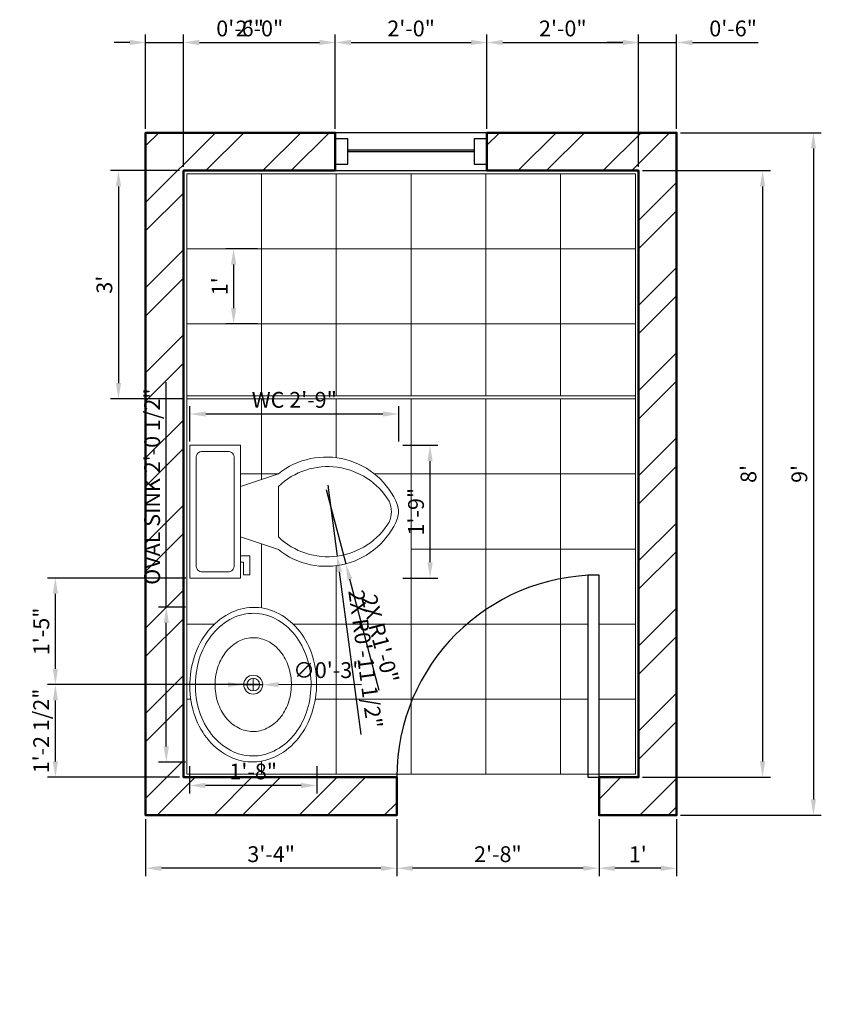
# Model space of a CAD drawing. Units: inches. Extents: x 3082 to 3209, y 1055 to 1366.
# Tile 2 of 2: x 3082 to 3209, y 1210 to 1366. Entities that reach past the tile are written whole.
import ezdxf

# ---------------------------------------------------------------- set-up
doc = ezdxf.new("R2010")
doc.units = ezdxf.units.IN
for name, color, linetype, lineweight in [('A-ANNO-DIMS', 2, 'Continuous', 18), ('A-DOOR', 3, 'Continuous', 25), ('A-FLOR-FIXT', 9, 'Continuous', 18), ('A-FLOR-PATT', 252, 'Continuous', 13), ('A-GLAZ', 4, 'Continuous', 25), ('A-WALL', 7, 'Continuous', 50), ('A-WALL-PATT', 8, 'Continuous', 13)]:
    doc.layers.add(name, color=color, linetype=linetype, lineweight=lineweight)
doc.styles.get("Standard").update_dxf_attribs({"font": 'arial.ttf'})
doc.dimstyles.new('ISO-25', dxfattribs={"dimtxt": 2.5, "dimasz": 2.5, "dimexe": 1.25, "dimexo": 0.625, "dimtad": 1, "dimdec": 0, "dimlunit": 3, "dimtxsty": 'Standard', "dimcen": 2.5, "dimadec": 0, "dimazin": 0, "dimtfac": 1, "dimtdec": 0, "dimtmove": 0, "dimatfit": 3, "dimfxl": 1, "dimarcsym": 0})

# ---------------------------------------------------------------- blocks, each defined once
blk = doc.blocks.new('*U2')
for p, q in [((0, 0), (0, -6)), ((-32, 0), (-32, -6))]:
    blk.add_line(p, q)
blk.add_lwpolyline([(0, 0), (0, 32), (-1.75, 32), (-1.75, 0)], close=True)
blk.add_arc((0, 0), 32, 90, 180)
blk = doc.blocks.new('Toilet - top')
for p, q in [((9.5, -6), (9.5, -2)), ((-10, -8.5), (-8, -8.5)), ((-10, -9.5), (-10, -8.5)), ((-8, -8.5), (-8, -8)), ((-7, -8), (-7, -9.5)), ((-4, -8), (-6, -14)), ((4, -8), (6, -14)), ((-7, -9.5), (-10, -9.5)), ((4, -14), (-4, -14))]:
    blk.add_line(p, q)
blk.add_lwpolyline([(10.5, -8), (10.5, 0), (-10.5, 0), (-10.5, -8)], close=True)
for points in [[(8.5, -1), (-8.5, -1)], [(-9.5, -2), (-9.5, -6)], [(-8.5, -7), (8.5, -7)]]:
    blk.add_lwpolyline(points)
for centre, radius, start, end in [((-8.62, -1.88), 0.884, 81.8699, 188.1301), ((8.62, -1.88), 0.884, 351.8699, 98.1301), ((-8.62, -6.12), 0.884, 171.8699, 278.1301), ((8.62, -6.12), 0.884, 261.8699, 8.1301), ((3.52, -21.58), 12.17, 141.4691, 247.9714), ((4.2, -21.82), 11.33, 136.3677, 238.9468), ((-3.52, -21.58), 12.17, 292.0284, 38.5307), ((-4.2, -21.82), 11.33, 301.053, 43.6321), ((0, -27.88), 4, 245.7318, 294.2682), ((0, -29), 4, 254.8605, 285.1395)]:
    blk.add_arc(centre, radius, start, end)
blk = doc.blocks.new('Sink - Oval top')
for p, q in [((-1, 0), (1, 0)), ((0, 1), (0, -1))]:
    blk.add_line(p, q)
for points in [[(-12.23, 0.39, 0.117634), (-11.46, -3.36, 0.104469), (-8.88, -6.8, 0.090016), (-5.08, -9.07, 0.08192), (-0.32, -10.02, 0.08192), (4.49, -9.38, 0.090016), (8.42, -7.36, 0.104469), (11.22, -4.09, 0.117634), (12.23, -0.39, 0.117634), (11.46, 3.36, 0.104469), (8.88, 6.8, 0.090016), (5.08, 9.07, 0.08192), (0.32, 10.02, 0.08192), (-4.49, 9.38, 0.090016), (-8.42, 7.36, 0.104469), (-11.22, 4.09, 0.117634)], [(-11.29, 0.16, 0.118622), (-10.52, -3.25, 0.104678), (-8.07, -6.36, 0.089562), (-4.54, -8.37, 0.081185), (-0.13, -9.15, 0.081185), (4.3, -8.49, 0.089562), (7.89, -6.58, 0.104678), (10.42, -3.55, 0.118622), (11.29, -0.16, 0.118622), (10.52, 3.25, 0.104678), (8.07, 6.36, 0.089562), (4.54, 8.37, 0.081185), (0.13, 9.15, 0.081185), (-4.3, 8.49, 0.089562), (-7.89, 6.58, 0.104678), (-10.42, 3.55, 0.118622)], [(-7.42, 0.08, 0.118283), (-6.91, -2.17, 0.104607), (-5.29, -4.21, 0.089718), (-2.97, -5.53, 0.081436), (-0.07, -6.04, 0.081436), (2.84, -5.59, 0.089718), (5.2, -4.33, 0.104607), (6.86, -2.32, 0.118283), (7.42, -0.08, 0.118283), (6.91, 2.17, 0.104607), (5.29, 4.21, 0.089718), (2.97, 5.53, 0.081436), (0.07, 6.04, 0.081436), (-2.84, 5.59, 0.089718), (-5.2, 4.33, 0.104607), (-6.86, 2.32, 0.118283)]]:
    blk.add_lwpolyline(points, format="xyb", close=True)
for radius in [1.5, 1]:
    blk.add_circle((0, 0), radius)
blk = doc.blocks.new('*D7')
at = {"layer": 'A-ANNO-DIMS', "color": 0, "lineweight": -2, "transparency": 16777216}
for p, q in [((3186.42, 1348.24), (3208.7, 1348.24)), ((3207.45, 1345.74), (3207.45, 1242.74)), ((3186.42, 1240.24), (3208.7, 1240.24))]:
    blk.add_line(p, q, dxfattribs=at)
at = {"layer": 'A-ANNO-DIMS', "color": 0, "transparency": 16777216}
for points in [[(3207.03, 1345.74), (3207.86, 1345.74), (3207.45, 1348.24)], [(3207.03, 1242.74), (3207.86, 1242.74), (3207.45, 1240.24)]]:
    blk.add_solid(points, dxfattribs=at)
at = {"layer": 'Defpoints', "color": 0, "transparency": 16777216}
for p in [(3185.8, 1348.24), (3185.8, 1240.24), (3207.45, 1240.24)]:
    blk.add_point(p, dxfattribs=at)
at = {"layer": 'A-ANNO-DIMS', "color": 0, "transparency": 16777216, "insert": (3205.55, 1294.24), "char_height": 2.5, "attachment_point": 5, "rotation": 90}
blk.add_mtext("9'", dxfattribs=at)
blk = doc.blocks.new('*D8')
at = {"layer": 'A-ANNO-DIMS', "color": 0, "lineweight": -2, "transparency": 16777216}
for p, q in [((3180.42, 1342.24), (3200.66, 1342.24)), ((3199.41, 1339.74), (3199.41, 1248.74)), ((3180.42, 1246.24), (3200.66, 1246.24))]:
    blk.add_line(p, q, dxfattribs=at)
at = {"layer": 'A-ANNO-DIMS', "color": 0, "transparency": 16777216}
for points in [[(3198.99, 1339.74), (3199.82, 1339.74), (3199.41, 1342.24)], [(3198.99, 1248.74), (3199.82, 1248.74), (3199.41, 1246.24)]]:
    blk.add_solid(points, dxfattribs=at)
at = {"layer": 'Defpoints', "color": 0, "transparency": 16777216}
for p in [(3179.8, 1342.24), (3179.8, 1246.24), (3199.41, 1246.24)]:
    blk.add_point(p, dxfattribs=at)
at = {"layer": 'A-ANNO-DIMS', "color": 0, "transparency": 16777216, "insert": (3197.5, 1294.24), "char_height": 2.5, "attachment_point": 5, "rotation": 90}
blk.add_mtext("8'", dxfattribs=at)
blk = doc.blocks.new('*D9')
at = {"layer": 'A-ANNO-DIMS', "color": 0, "lineweight": -2, "transparency": 16777216}
for p, q in [((3173.53, 1239.61), (3173.53, 1230.6)), ((3185.8, 1239.61), (3185.8, 1230.6)), ((3183.3, 1231.85), (3176.03, 1231.85))]:
    blk.add_line(p, q, dxfattribs=at)
at = {"layer": 'A-ANNO-DIMS', "color": 0, "transparency": 16777216}
for points in [[(3176.03, 1232.26), (3176.03, 1231.43), (3173.53, 1231.85)], [(3183.3, 1232.26), (3183.3, 1231.43), (3185.8, 1231.85)]]:
    blk.add_solid(points, dxfattribs=at)
at = {"layer": 'Defpoints', "color": 0, "transparency": 16777216}
for p in [(3173.53, 1240.24), (3185.8, 1240.24), (3173.53, 1231.85)]:
    blk.add_point(p, dxfattribs=at)
at = {"layer": 'A-ANNO-DIMS', "color": 0, "transparency": 16777216, "insert": (3179.66, 1233.73), "char_height": 2.5, "attachment_point": 5}
blk.add_mtext("1'", dxfattribs=at)
blk = doc.blocks.new('*D10')
at = {"layer": 'A-ANNO-DIMS', "color": 0, "lineweight": -2, "transparency": 16777216}
for p, q in [((3141.53, 1239.61), (3141.53, 1230.6)), ((3173.53, 1239.61), (3173.53, 1230.6)), ((3171.03, 1231.85), (3144.03, 1231.85))]:
    blk.add_line(p, q, dxfattribs=at)
at = {"layer": 'A-ANNO-DIMS', "color": 0, "transparency": 16777216}
for points in [[(3144.03, 1232.26), (3144.03, 1231.43), (3141.53, 1231.85)], [(3171.03, 1232.26), (3171.03, 1231.43), (3173.53, 1231.85)]]:
    blk.add_solid(points, dxfattribs=at)
at = {"layer": 'Defpoints', "color": 0, "transparency": 16777216}
for p in [(3141.53, 1240.24), (3173.53, 1240.24), (3141.53, 1231.85)]:
    blk.add_point(p, dxfattribs=at)
at = {"layer": 'A-ANNO-DIMS', "color": 0, "transparency": 16777216, "insert": (3157.53, 1233.75), "char_height": 2.5, "attachment_point": 5}
blk.add_mtext('2\'-8"', dxfattribs=at)
blk = doc.blocks.new('*D11')
at = {"layer": 'A-ANNO-DIMS', "color": 0, "lineweight": -2, "transparency": 16777216}
for p, q in [((3101.8, 1239.61), (3101.8, 1230.6)), ((3141.53, 1239.61), (3141.53, 1230.6)), ((3139.03, 1231.85), (3104.3, 1231.85))]:
    blk.add_line(p, q, dxfattribs=at)
at = {"layer": 'A-ANNO-DIMS', "color": 0, "transparency": 16777216}
for points in [[(3104.3, 1232.26), (3104.3, 1231.43), (3101.8, 1231.85)], [(3139.03, 1232.26), (3139.03, 1231.43), (3141.53, 1231.85)]]:
    blk.add_solid(points, dxfattribs=at)
at = {"layer": 'Defpoints', "color": 0, "transparency": 16777216}
for p in [(3101.8, 1240.24), (3141.53, 1240.24), (3101.8, 1231.85)]:
    blk.add_point(p, dxfattribs=at)
at = {"layer": 'A-ANNO-DIMS', "color": 0, "transparency": 16777216, "insert": (3121.66, 1233.75), "char_height": 2.5, "attachment_point": 5}
blk.add_mtext('3\'-4"', dxfattribs=at)
blk = doc.blocks.new('*D12')
at = {"layer": 'A-ANNO-DIMS', "color": 0, "lineweight": -2, "transparency": 16777216}
for p, q in [((3107.17, 1342.24), (3096.25, 1342.24)), ((3097.5, 1339.74), (3097.5, 1308.61)), ((3107.67, 1306.11), (3096.25, 1306.11))]:
    blk.add_line(p, q, dxfattribs=at)
at = {"layer": 'A-ANNO-DIMS', "color": 0, "transparency": 16777216}
for points in [[(3097.09, 1339.74), (3097.92, 1339.74), (3097.5, 1342.24)], [(3097.09, 1308.61), (3097.92, 1308.61), (3097.5, 1306.11)]]:
    blk.add_solid(points, dxfattribs=at)
at = {"layer": 'Defpoints', "color": 0, "transparency": 16777216}
for p in [(3107.8, 1342.24), (3097.5, 1306.11), (3108.3, 1306.11)]:
    blk.add_point(p, dxfattribs=at)
at = {"layer": 'A-ANNO-DIMS', "color": 0, "transparency": 16777216, "insert": (3095.6, 1324.18), "char_height": 2.5, "attachment_point": 5, "rotation": 90}
blk.add_mtext("3'", dxfattribs=at)
blk = doc.blocks.new('*D13')
at = {"layer": 'A-ANNO-DIMS', "color": 0, "lineweight": -2, "transparency": 16777216}
for p, q in [((3119.51, 1329.86), (3114.47, 1329.86)), ((3115.72, 1327.36), (3115.72, 1320.49)), ((3119.51, 1317.99), (3114.47, 1317.99))]:
    blk.add_line(p, q, dxfattribs=at)
at = {"layer": 'A-ANNO-DIMS', "color": 0, "transparency": 16777216}
for points in [[(3115.3, 1327.36), (3116.14, 1327.36), (3115.72, 1329.86)], [(3115.3, 1320.49), (3116.14, 1320.49), (3115.72, 1317.99)]]:
    blk.add_solid(points, dxfattribs=at)
at = {"layer": 'Defpoints', "color": 0, "transparency": 16777216}
for p in [(3120.13, 1329.86), (3115.72, 1317.99), (3120.13, 1317.99)]:
    blk.add_point(p, dxfattribs=at)
at = {"layer": 'A-ANNO-DIMS', "color": 0, "transparency": 16777216, "insert": (3113.84, 1323.93), "char_height": 2.5, "attachment_point": 5, "rotation": 90}
blk.add_mtext("1'", dxfattribs=at)
blk = doc.blocks.new('*D18')
at = {"layer": 'A-ANNO-DIMS', "color": 0, "lineweight": -2, "transparency": 16777216}
for p, q in [((3108.8, 1299.39), (3108.8, 1304.97)), ((3141.84, 1299.39), (3141.84, 1304.97)), ((3139.34, 1303.72), (3111.3, 1303.72))]:
    blk.add_line(p, q, dxfattribs=at)
at = {"layer": 'A-ANNO-DIMS', "color": 0, "transparency": 16777216}
for points in [[(3111.3, 1304.14), (3111.3, 1303.31), (3108.8, 1303.72)], [(3139.34, 1304.14), (3139.34, 1303.31), (3141.84, 1303.72)]]:
    blk.add_solid(points, dxfattribs=at)
at = {"layer": 'Defpoints', "color": 0, "transparency": 16777216}
for p in [(3108.8, 1303.72), (3108.8, 1298.77), (3141.84, 1298.77)]:
    blk.add_point(p, dxfattribs=at)
at = {"layer": 'A-ANNO-DIMS', "color": 0, "transparency": 16777216, "insert": (3125.32, 1305.64), "char_height": 2.5, "attachment_point": 5}
blk.add_mtext('WC 2\'-9"', dxfattribs=at)
blk = doc.blocks.new('*D19')
at = {"layer": 'A-ANNO-DIMS', "color": 0, "lineweight": -2, "transparency": 16777216}
for p, q in [((3142.47, 1298.77), (3148.05, 1298.77)), ((3146.8, 1280.27), (3146.8, 1296.27)), ((3142.47, 1277.77), (3148.05, 1277.77))]:
    blk.add_line(p, q, dxfattribs=at)
at = {"layer": 'A-ANNO-DIMS', "color": 0, "transparency": 16777216}
for points in [[(3146.38, 1296.27), (3147.22, 1296.27), (3146.8, 1298.77)], [(3146.38, 1280.27), (3147.22, 1280.27), (3146.8, 1277.77)]]:
    blk.add_solid(points, dxfattribs=at)
at = {"layer": 'Defpoints', "color": 0, "transparency": 16777216}
for p in [(3141.84, 1298.77), (3146.8, 1298.77), (3141.84, 1277.77)]:
    blk.add_point(p, dxfattribs=at)
at = {"layer": 'A-ANNO-DIMS', "color": 0, "transparency": 16777216, "insert": (3144.9, 1288.27), "char_height": 2.5, "attachment_point": 5, "rotation": 90}
blk.add_mtext('1\'-9"', dxfattribs=at)
blk = doc.blocks.new('*D20')
at = {"layer": 'A-ANNO-DIMS', "color": 0, "lineweight": -2, "transparency": 16777216}
for p, q in [((3105.07, 1273.17), (3105.07, 1308.78)), ((3108.13, 1273.17), (3103.82, 1273.17)), ((3105.07, 1251.12), (3105.07, 1270.67)), ((3108.13, 1248.62), (3103.82, 1248.62))]:
    blk.add_line(p, q, dxfattribs=at)
at = {"layer": 'A-ANNO-DIMS', "color": 0, "transparency": 16777216}
for points in [[(3104.65, 1270.67), (3105.49, 1270.67), (3105.07, 1273.17)], [(3104.65, 1251.12), (3105.49, 1251.12), (3105.07, 1248.62)]]:
    blk.add_solid(points, dxfattribs=at)
at = {"layer": 'Defpoints', "color": 0, "transparency": 16777216}
for p in [(3105.07, 1273.17), (3108.75, 1273.17), (3108.75, 1248.62)]:
    blk.add_point(p, dxfattribs=at)
at = {"layer": 'A-ANNO-DIMS', "color": 0, "transparency": 16777216, "insert": (3103.15, 1292.23), "char_height": 2.5, "attachment_point": 5, "rotation": 90}
blk.add_mtext('OVAL SINK 2\'-0 1/2"', dxfattribs=at)
blk = doc.blocks.new('*D21')
at = {"layer": 'A-ANNO-DIMS', "color": 0, "lineweight": -2, "transparency": 16777216}
for p, q in [((3108.75, 1248), (3108.75, 1243.69)), ((3128.89, 1248), (3128.89, 1243.69)), ((3126.39, 1244.94), (3111.25, 1244.94))]:
    blk.add_line(p, q, dxfattribs=at)
at = {"layer": 'A-ANNO-DIMS', "color": 0, "transparency": 16777216}
for points in [[(3111.25, 1245.36), (3111.25, 1244.52), (3108.75, 1244.94)], [(3126.39, 1245.36), (3126.39, 1244.52), (3128.89, 1244.94)]]:
    blk.add_solid(points, dxfattribs=at)
at = {"layer": 'Defpoints', "color": 0, "transparency": 16777216}
for p in [(3108.75, 1248.62), (3128.89, 1248.62), (3108.75, 1244.94)]:
    blk.add_point(p, dxfattribs=at)
at = {"layer": 'A-ANNO-DIMS', "color": 0, "transparency": 16777216, "insert": (3118.82, 1246.84), "char_height": 2.5, "attachment_point": 5}
blk.add_mtext('1\'-8"', dxfattribs=at)
blk = doc.blocks.new('*D24')
at = {"layer": 'A-ANNO-DIMS', "color": 0, "lineweight": -2, "transparency": 16777216}
for p, q in [((3101.8, 1348.86), (3101.8, 1363.76)), ((3107.8, 1342.86), (3107.8, 1363.76)), ((3099.3, 1362.51), (3096.8, 1362.51)), ((3101.8, 1362.51), (3107.8, 1362.51)), ((3110.3, 1362.51), (3120.69, 1362.51))]:
    blk.add_line(p, q, dxfattribs=at)
at = {"layer": 'A-ANNO-DIMS', "color": 0, "transparency": 16777216}
for points in [[(3099.3, 1362.93), (3099.3, 1362.1), (3101.8, 1362.51)], [(3110.3, 1362.93), (3110.3, 1362.1), (3107.8, 1362.51)]]:
    blk.add_solid(points, dxfattribs=at)
at = {"layer": 'Defpoints', "color": 0, "transparency": 16777216}
for p in [(3107.8, 1362.51), (3101.8, 1348.24), (3107.8, 1342.24)]:
    blk.add_point(p, dxfattribs=at)
at = {"layer": 'A-ANNO-DIMS', "color": 0, "transparency": 16777216, "insert": (3116.74, 1364.41), "char_height": 2.5, "attachment_point": 5}
blk.add_mtext('0\'-6"', dxfattribs=at)
blk = doc.blocks.new('*D25')
at = {"layer": 'A-ANNO-DIMS', "color": 0, "lineweight": -2, "transparency": 16777216}
for p, q in [((3107.8, 1342.86), (3107.8, 1363.76)), ((3131.8, 1348.86), (3131.8, 1363.76)), ((3110.3, 1362.51), (3129.3, 1362.51))]:
    blk.add_line(p, q, dxfattribs=at)
at = {"layer": 'A-ANNO-DIMS', "color": 0, "transparency": 16777216}
for points in [[(3110.3, 1362.93), (3110.3, 1362.1), (3107.8, 1362.51)], [(3129.3, 1362.93), (3129.3, 1362.1), (3131.8, 1362.51)]]:
    blk.add_solid(points, dxfattribs=at)
at = {"layer": 'Defpoints', "color": 0, "transparency": 16777216}
for p in [(3131.8, 1362.51), (3131.8, 1348.24), (3107.8, 1342.24)]:
    blk.add_point(p, dxfattribs=at)
at = {"layer": 'A-ANNO-DIMS', "color": 0, "transparency": 16777216, "insert": (3119.8, 1364.41), "char_height": 2.5, "attachment_point": 5}
blk.add_mtext('2\'-0"', dxfattribs=at)
blk = doc.blocks.new('*D26')
at = {"layer": 'A-ANNO-DIMS', "color": 0, "lineweight": -2, "transparency": 16777216}
for p, q in [((3131.8, 1348.86), (3131.8, 1363.76)), ((3155.8, 1348.86), (3155.8, 1363.76)), ((3134.3, 1362.51), (3153.3, 1362.51))]:
    blk.add_line(p, q, dxfattribs=at)
at = {"layer": 'A-ANNO-DIMS', "color": 0, "transparency": 16777216}
for points in [[(3134.3, 1362.93), (3134.3, 1362.1), (3131.8, 1362.51)], [(3153.3, 1362.93), (3153.3, 1362.1), (3155.8, 1362.51)]]:
    blk.add_solid(points, dxfattribs=at)
at = {"layer": 'Defpoints', "color": 0, "transparency": 16777216}
for p in [(3155.8, 1362.51), (3131.8, 1348.24), (3155.8, 1348.24)]:
    blk.add_point(p, dxfattribs=at)
at = {"layer": 'A-ANNO-DIMS', "color": 0, "transparency": 16777216, "insert": (3143.8, 1364.41), "char_height": 2.5, "attachment_point": 5}
blk.add_mtext('2\'-0"', dxfattribs=at)
blk = doc.blocks.new('*D27')
at = {"layer": 'A-ANNO-DIMS', "color": 0, "lineweight": -2, "transparency": 16777216}
for p, q in [((3155.8, 1348.86), (3155.8, 1363.76)), ((3179.8, 1342.86), (3179.8, 1363.76)), ((3158.3, 1362.51), (3177.3, 1362.51))]:
    blk.add_line(p, q, dxfattribs=at)
at = {"layer": 'A-ANNO-DIMS', "color": 0, "transparency": 16777216}
for points in [[(3158.3, 1362.93), (3158.3, 1362.1), (3155.8, 1362.51)], [(3177.3, 1362.93), (3177.3, 1362.1), (3179.8, 1362.51)]]:
    blk.add_solid(points, dxfattribs=at)
at = {"layer": 'Defpoints', "color": 0, "transparency": 16777216}
for p in [(3179.8, 1362.51), (3155.8, 1348.24), (3179.8, 1342.24)]:
    blk.add_point(p, dxfattribs=at)
at = {"layer": 'A-ANNO-DIMS', "color": 0, "transparency": 16777216, "insert": (3167.8, 1364.41), "char_height": 2.5, "attachment_point": 5}
blk.add_mtext('2\'-0"', dxfattribs=at)
blk = doc.blocks.new('*D28')
at = {"layer": 'A-ANNO-DIMS', "color": 0, "lineweight": -2, "transparency": 16777216}
for p, q in [((3179.8, 1342.86), (3179.8, 1363.76)), ((3185.8, 1348.86), (3185.8, 1363.76)), ((3177.3, 1362.51), (3174.8, 1362.51)), ((3179.8, 1362.51), (3185.8, 1362.51)), ((3188.3, 1362.51), (3198.69, 1362.51))]:
    blk.add_line(p, q, dxfattribs=at)
at = {"layer": 'A-ANNO-DIMS', "color": 0, "transparency": 16777216}
for points in [[(3177.3, 1362.93), (3177.3, 1362.1), (3179.8, 1362.51)], [(3188.3, 1362.93), (3188.3, 1362.1), (3185.8, 1362.51)]]:
    blk.add_solid(points, dxfattribs=at)
at = {"layer": 'Defpoints', "color": 0, "transparency": 16777216}
for p in [(3185.8, 1362.51), (3185.8, 1348.24), (3179.8, 1342.24)]:
    blk.add_point(p, dxfattribs=at)
at = {"layer": 'A-ANNO-DIMS', "color": 0, "transparency": 16777216, "insert": (3194.74, 1364.41), "char_height": 2.5, "attachment_point": 5}
blk.add_mtext('0\'-6"', dxfattribs=at)
blk = doc.blocks.new('*D29')
at = {"layer": 'A-ANNO-DIMS', "color": 0, "lineweight": -2, "transparency": 16777216}
for p, q in [((3119.7, 1260.9), (3086.27, 1260.9)), ((3087.52, 1248.74), (3087.52, 1258.4)), ((3107.17, 1246.24), (3086.27, 1246.24))]:
    blk.add_line(p, q, dxfattribs=at)
at = {"layer": 'A-ANNO-DIMS', "color": 0, "transparency": 16777216}
for points in [[(3087.11, 1258.4), (3087.94, 1258.4), (3087.52, 1260.9)], [(3087.11, 1248.74), (3087.94, 1248.74), (3087.52, 1246.24)]]:
    blk.add_solid(points, dxfattribs=at)
at = {"layer": 'Defpoints', "color": 0, "transparency": 16777216}
for p in [(3087.52, 1260.9), (3120.32, 1260.9), (3107.8, 1246.24)]:
    blk.add_point(p, dxfattribs=at)
at = {"layer": 'A-ANNO-DIMS', "color": 0, "transparency": 16777216, "insert": (3085.6, 1253.57), "char_height": 2.5, "attachment_point": 5, "rotation": 90}
blk.add_mtext('1\'-2 1/2"', dxfattribs=at)
blk = doc.blocks.new('*D30')
at = {"layer": 'A-ANNO-DIMS', "color": 0, "lineweight": -2, "transparency": 16777216}
for p, q in [((3108.17, 1277.77), (3086.27, 1277.77)), ((3087.52, 1263.4), (3087.52, 1275.27)), ((3119.7, 1260.9), (3086.27, 1260.9))]:
    blk.add_line(p, q, dxfattribs=at)
at = {"layer": 'A-ANNO-DIMS', "color": 0, "transparency": 16777216}
for points in [[(3087.11, 1275.27), (3087.94, 1275.27), (3087.52, 1277.77)], [(3087.11, 1263.4), (3087.94, 1263.4), (3087.52, 1260.9)]]:
    blk.add_solid(points, dxfattribs=at)
at = {"layer": 'Defpoints', "color": 0, "transparency": 16777216}
for p in [(3087.52, 1277.77), (3108.8, 1277.77), (3120.32, 1260.9)]:
    blk.add_point(p, dxfattribs=at)
at = {"layer": 'A-ANNO-DIMS', "color": 0, "transparency": 16777216, "insert": (3085.62, 1269.33), "char_height": 2.5, "attachment_point": 5, "rotation": 90}
blk.add_mtext('1\'-5"', dxfattribs=at)
blk = doc.blocks.new('*D41')
at = {"layer": 'A-ANNO-DIMS', "color": 0, "lineweight": -2, "transparency": 16777216}
for p, q in [((3130.38, 1291.79), (3133.47, 1280.02)), ((3138.73, 1259.99), (3134.11, 1277.6))]:
    blk.add_line(p, q, dxfattribs=at)
at = {"layer": 'A-ANNO-DIMS', "color": 0, "transparency": 16777216}
blk.add_solid([(3134.51, 1277.7), (3133.7, 1277.49), (3133.47, 1280.02)], dxfattribs=at)
at = {"layer": 'Defpoints', "color": 0, "transparency": 16777216}
for p in [(3130.38, 1291.79), (3133.47, 1280.02)]:
    blk.add_point(p, dxfattribs=at)
at = {"layer": 'A-ANNO-DIMS', "color": 0, "transparency": 16777216, "insert": (3138.57, 1268.07), "char_height": 2.5, "attachment_point": 5, "rotation": 284.7218}
blk.add_mtext('2X R1\'-0"', dxfattribs=at)
blk = doc.blocks.new('*D42')
at = {"layer": 'A-ANNO-DIMS', "color": 0, "lineweight": -2, "transparency": 16777216}
for p, q in [((3130.61, 1292.47), (3132.12, 1281.24)), ((3135.92, 1253.02), (3132.46, 1278.76))]:
    blk.add_line(p, q, dxfattribs=at)
at = {"layer": 'A-ANNO-DIMS', "color": 0, "transparency": 16777216}
blk.add_solid([(3132.87, 1278.82), (3132.04, 1278.71), (3132.12, 1281.24)], dxfattribs=at)
at = {"layer": 'Defpoints', "color": 0, "transparency": 16777216}
for p in [(3130.61, 1292.47), (3132.12, 1281.24)]:
    blk.add_point(p, dxfattribs=at)
at = {"layer": 'A-ANNO-DIMS', "color": 0, "transparency": 16777216, "insert": (3136.25, 1264.91), "char_height": 2.5, "attachment_point": 5, "rotation": 277.6572}
blk.add_mtext('2X R0\'-11 1/2"', dxfattribs=at)
blk = doc.blocks.new('*D43')
at = {"layer": 'A-ANNO-DIMS', "color": 0, "lineweight": -2, "transparency": 16777216}
for p, q in [((3114.82, 1260.9), (3112.32, 1260.9)), ((3117.32, 1260.9), (3120.32, 1260.9)), ((3135.94, 1260.89), (3122.82, 1260.9))]:
    blk.add_line(p, q, dxfattribs=at)
at = {"layer": 'A-ANNO-DIMS', "color": 0, "transparency": 16777216}
for points in [[(3114.82, 1261.32), (3114.82, 1260.48), (3117.32, 1260.9)], [(3122.82, 1261.31), (3122.82, 1260.48), (3120.32, 1260.9)]]:
    blk.add_solid(points, dxfattribs=at)
at = {"layer": 'Defpoints', "color": 0, "transparency": 16777216}
for p in [(3117.32, 1260.9), (3120.32, 1260.9)]:
    blk.add_point(p, dxfattribs=at)
at = {"layer": 'A-ANNO-DIMS', "color": 0, "transparency": 16777216, "insert": (3130.63, 1262.87), "char_height": 2.5, "attachment_point": 5, "rotation": 359.9824}
blk.add_mtext('∅0\'-3"', dxfattribs=at)

msp = doc.modelspace()

# ---------------------------------------------------------------- hatches: boundary and pattern name
at = {"layer": 'A-WALL-PATT'}
h = msp.add_hatch(dxfattribs=at)
h.set_pattern_fill('ANSI32', color=256)
h.paths.add_polyline_path([(3185.8, 1196.04), (3101.8, 1196.04), (3101.8, 1076.04), (3109.8, 1076.04), (3109.8, 1160.04), (3109.8, 1190.04), (3179.8, 1190.04), (3179.8, 1076.04), (3185.8, 1076.04)])
h.paths.add_polyline_path([(3185.8, 1348.24), (3155.8, 1348.24), (3155.8, 1342.24), (3179.8, 1342.24), (3179.8, 1246.24), (3173.53, 1246.24), (3173.53, 1240.24), (3185.8, 1240.24)])
h.paths.add_polyline_path([(3107.8, 1342.24), (3131.8, 1342.24), (3131.8, 1348.24), (3101.8, 1348.24), (3101.8, 1240.24), (3141.53, 1240.24), (3141.53, 1246.24), (3107.8, 1246.24)])

# ---------------------------------------------------------------- linework, layer by layer
at = {"layer": 'A-FLOR-PATT', "transparency": 33554569}
for p, q in [((3179.3, 1341.74), (3108.3, 1341.74)), ((3108.3, 1341.74), (3108.3, 1246.74)), ((3120.13, 1341.74), (3120.13, 1306.61)), ((3131.96, 1341.74), (3131.96, 1306.61)), ((3143.8, 1341.74), (3143.8, 1306.61)), ((3155.63, 1341.74), (3155.63, 1306.61)), ((3167.46, 1341.74), (3167.46, 1306.61)), ((3179.3, 1329.86), (3108.3, 1329.86)), ((3179.3, 1317.99), (3108.3, 1317.99)), ((3179.3, 1306.11), (3108.3, 1306.11)), ((3120.13, 1306.11), (3120.13, 1293.38)), ((3131.96, 1306.11), (3131.96, 1296.81)), ((3143.8, 1306.11), (3143.8, 1246.74)), ((3155.63, 1306.11), (3155.63, 1246.74)), ((3167.46, 1306.11), (3167.46, 1246.74)), ((3122.71, 1294.24), (3116.8, 1294.24)), ((3179.3, 1294.24), (3137.99, 1294.24)), ((3120.13, 1283.16), (3120.13, 1273.05)), ((3179.3, 1282.36), (3143.8, 1282.36)), ((3131.96, 1279.72), (3131.96, 1246.74)), ((3112.7, 1270.49), (3108.3, 1270.49)), ((3171.78, 1270.49), (3125.14, 1270.49)), ((3179.3, 1270.49), (3173.53, 1270.49)), ((3108.95, 1258.61), (3108.3, 1258.61)), ((3171.78, 1258.61), (3128.64, 1258.61)), ((3179.3, 1258.61), (3173.53, 1258.61)), ((3120.13, 1248.79), (3120.13, 1246.74))]:
    msp.add_line(p, q, dxfattribs=at)
at = {"layer": 'A-FLOR-PATT'}
for p, q in [((3179.3, 1306.61), (3108.3, 1306.61)), ((3179.3, 1306.11), (3108.3, 1306.11))]:
    msp.add_line(p, q, dxfattribs=at)
msp.add_lwpolyline([(3108.3, 1341.74), (3108.3, 1246.74), (3141.53, 1246.74), (3141.53, 1246.24), (3107.8, 1246.24), (3107.8, 1342.24), (3179.8, 1342.24), (3179.8, 1246.24), (3173.53, 1246.24), (3173.53, 1246.74), (3179.3, 1246.74), (3179.3, 1341.74)], close=True, dxfattribs=at)
at = {"layer": 'A-FLOR-PATT', "transparency": 33554569}
msp.add_lwpolyline([(3179.3, 1246.74), (3179.3, 1341.74), (3179.3, 1246.74), (3108.3, 1246.74)], close=True, dxfattribs=at)
at = {"layer": 'A-FLOR-PATT'}
msp.add_lwpolyline([(3108.3, 1306.11), (3108.3, 1341.74), (3179.3, 1341.74), (3179.3, 1306.11)], dxfattribs=at)
at = {"layer": 'A-GLAZ'}
for points in [[(3131.8, 1342.24), (3155.8, 1342.24), (3155.8, 1348.24), (3131.8, 1348.24)], [(3131.8, 1343.24), (3133.8, 1343.24), (3133.8, 1347.24), (3131.8, 1347.24)], [(3153.8, 1343.24), (3155.8, 1343.24), (3155.8, 1347.24), (3153.8, 1347.24)], [(3133.8, 1345.24), (3153.8, 1345.24), (3153.8, 1345.49), (3133.8, 1345.49)]]:
    msp.add_lwpolyline(points, close=True, dxfattribs=at)
at = {"layer": 'A-WALL'}
for points in [[(3131.8, 1342.24), (3107.8, 1342.24), (3107.8, 1246.24), (3141.53, 1246.24), (3141.53, 1240.24), (3101.8, 1240.24), (3101.8, 1348.24), (3131.8, 1348.24)], [(3155.8, 1348.24), (3185.8, 1348.24), (3185.8, 1240.24), (3173.53, 1240.24), (3173.53, 1246.24), (3179.8, 1246.24), (3179.8, 1342.24), (3155.8, 1342.24)]]:
    msp.add_lwpolyline(points, close=True, dxfattribs=at)

# ---------------------------------------------------------------- block references
at = {"layer": 'A-DOOR'}
msp.add_blockref('*U2', (3173.53, 1246.24), dxfattribs=at)
at = {"layer": 'A-FLOR-FIXT', "rotation": 90}
for name, p in [('Toilet - top', (3108.8, 1288.27)), ('Sink - Oval top', (3118.82, 1260.9))]:
    msp.add_blockref(name, p, dxfattribs=at)

# ---------------------------------------------------------------- dimensions: what is measured, and where the dimension line sits
at = {"layer": 'A-ANNO-DIMS'}
for base, p1, p2, override, picture, middle in [((3107.8, 1362.51), (3101.8, 1348.24), (3107.8, 1342.24), {"dimdec": 1, "dimlfac": 1, "dimrnd": 0, "dimzin": 1, "dimdsep": 46, "dimlunit": 4, "dimfrac": 2}, '*D24', (3116.74, 1364.41)), ((3131.8, 1362.51), (3107.8, 1342.24), (3131.8, 1348.24), {"dimdec": 1, "dimlfac": 1, "dimrnd": 0, "dimzin": 1, "dimdsep": 46, "dimlunit": 4, "dimfrac": 2}, '*D25', (3119.8, 1364.41)), ((3155.8, 1362.51), (3131.8, 1348.24), (3155.8, 1348.24), {"dimdec": 1, "dimlfac": 1, "dimrnd": 0, "dimzin": 1, "dimdsep": 46, "dimlunit": 4, "dimfrac": 2}, '*D26', (3143.8, 1364.41)), ((3179.8, 1362.51), (3155.8, 1348.24), (3179.8, 1342.24), {"dimdec": 1, "dimlfac": 1, "dimrnd": 0, "dimzin": 1, "dimdsep": 46, "dimlunit": 4, "dimfrac": 2}, '*D27', (3167.8, 1364.41)), ((3185.8, 1362.51), (3179.8, 1342.24), (3185.8, 1348.24), {"dimdec": 1, "dimlfac": 1, "dimrnd": 0, "dimzin": 1, "dimdsep": 46, "dimlunit": 4, "dimfrac": 2}, '*D28', (3194.74, 1364.41)), ((3101.8, 1231.85), (3141.53, 1240.24), (3101.8, 1240.24), {"dimclrd": 0, "dimclre": 0, "dimclrt": 0, "dimtmove": 1}, '*D11', (3121.66, 1233.75)), ((3141.53, 1231.85), (3173.53, 1240.24), (3141.53, 1240.24), {"dimclrd": 0, "dimclre": 0, "dimclrt": 0, "dimtmove": 1}, '*D10', (3157.53, 1233.75)), ((3173.53, 1231.85), (3185.8, 1240.24), (3173.53, 1240.24), {"dimclrd": 0, "dimclre": 0, "dimclrt": 0}, '*D9', (3179.66, 1233.73))]:
    dim = msp.add_linear_dim(base=base, p1=p1, p2=p2, dimstyle='ISO-25', override=override, dxfattribs=at)
    dim.commit()
    dim.dimension.update_dxf_attribs({"geometry": picture, "text_midpoint": middle})
for base, p1, p2, angle, override, picture, middle in [((3207.45, 1240.24), (3185.8, 1348.24), (3185.8, 1240.24), 90, {"dimclrd": 0, "dimclre": 0, "dimclrt": 0}, '*D7', (3205.55, 1294.24)), ((3097.5, 1306.11), (3107.8, 1342.24), (3108.3, 1306.11), 90, {"dimclrd": 0, "dimclre": 0, "dimclrt": 0}, '*D12', (3095.6, 1324.18)), ((3199.41, 1246.24), (3179.8, 1342.24), (3179.8, 1246.24), 90, {"dimclrd": 0, "dimclre": 0, "dimclrt": 0}, '*D8', (3197.5, 1294.24)), ((3115.72, 1317.99), (3120.13, 1329.86), (3120.13, 1317.99), 90, {"dimclrd": 0, "dimclre": 0, "dimclrt": 0}, '*D13', (3113.84, 1323.93)), ((3146.8, 1298.77), (3141.84, 1277.77), (3141.84, 1298.77), 90, {"dimdec": 1, "dimrnd": 0, "dimzin": 1, "dimlunit": 4, "dimfrac": 2}, '*D19', (3144.9, 1288.27)), ((3087.52, 1277.77), (3120.32, 1260.9), (3108.8, 1277.77), 90, {"dimdec": 1, "dimlfac": 1, "dimrnd": 0, "dimzin": 1, "dimdsep": 46, "dimlunit": 4, "dimfrac": 2}, '*D30', (3085.62, 1269.33)), ((3087.52, 1260.9), (3107.8, 1246.24), (3120.32, 1260.9), 90, {"dimdec": 1, "dimlfac": 1, "dimrnd": 0, "dimzin": 1, "dimdsep": 46, "dimlunit": 4, "dimfrac": 2}, '*D29', (3085.6, 1253.57)), ((3108.75, 1244.94), (3128.89, 1248.62), (3108.75, 1248.62), 180, {"dimdec": 1, "dimrnd": 0, "dimzin": 1, "dimlunit": 4, "dimfrac": 2}, '*D21', (3118.82, 1246.84))]:
    dim = msp.add_linear_dim(base=base, p1=p1, p2=p2, angle=angle, dimstyle='ISO-25', override=override, dxfattribs=at)
    dim.commit()
    dim.dimension.update_dxf_attribs({"geometry": picture, "text_midpoint": middle})
for base, p1, p2, angle, text, picture, middle in [((3105.0697, 1273.1739), (3108.7523, 1248.623), (3108.7523, 1273.1739), 90, 'OVAL SINK <>', '*D20', (3103.1512, 1292.2275)), ((3108.8, 1303.72), (3141.84, 1298.77), (3108.8, 1298.77), 180, 'WC <>', '*D18', (3125.32, 1305.64))]:
    dim = msp.add_linear_dim(base=base, p1=p1, p2=p2, angle=angle, text=text, dimstyle='ISO-25', override={"dimdec": 1, "dimrnd": 0, "dimzin": 1, "dimlunit": 4, "dimfrac": 2}, dxfattribs=at)
    dim.commit()
    dim.dimension.update_dxf_attribs({"geometry": picture, "text_midpoint": middle})
for center, mpoint, picture, middle in [((3130.61, 1292.47), (3132.12, 1281.24), '*D42', (3136.25, 1264.91)), ((3130.38, 1291.79), (3133.47, 1280.02), '*D41', (3138.57, 1268.07))]:
    dim = msp.add_radius_dim(center=center, mpoint=mpoint, text='2X <>', dimstyle='ISO-25', override={"dimdec": 1, "dimlfac": 1, "dimrnd": 0, "dimzin": 1, "dimdsep": 46, "dimlunit": 4, "dimfrac": 2}, dxfattribs=at)
    dim.commit()
    dim.dimension.update_dxf_attribs({"geometry": picture, "text_midpoint": middle})
dim = msp.add_diameter_dim_2p(p1=(3117.32, 1260.9), p2=(3120.32, 1260.9), dimstyle='ISO-25', override={"dimdec": 1, "dimlfac": 1, "dimrnd": 0, "dimzin": 1, "dimdsep": 46, "dimlunit": 4, "dimfrac": 2}, dxfattribs=at)
dim.commit()
dim.dimension.update_dxf_attribs({"geometry": '*D43', "text_midpoint": (3130.63, 1260.89)})

doc.saveas('drawing.dxf')
